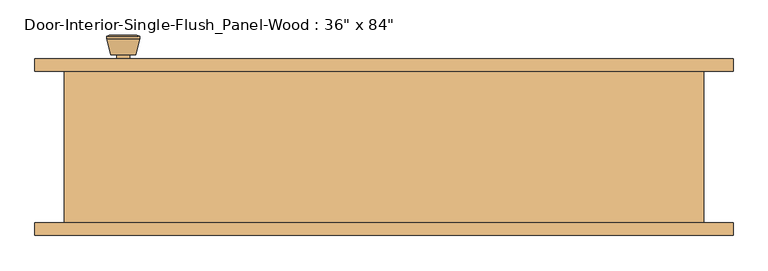
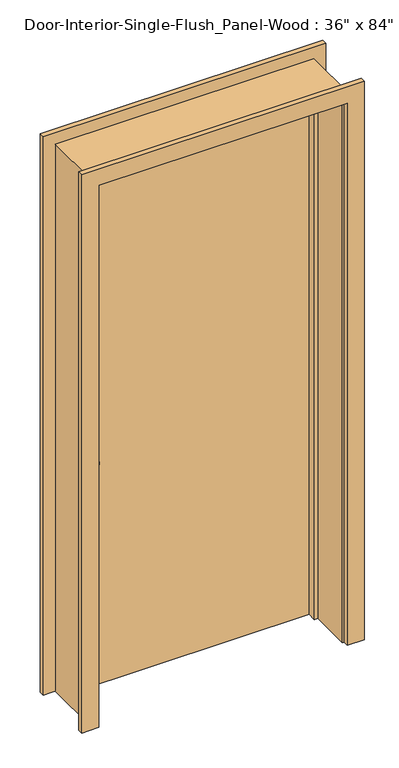
"""IFC4 building model written with IfcOpenShell, lengths in millimetres: door geometry."""

from ifc_helpers import new_model, si_unit, point, frame, frame_2d, origin, origin_with_axes, place, context, project, spatial, polyline, circle_curve, trimmed, segment, composite_curve, outline, extrude, faceted_brep, source, transform, mapped, element, save
from ifc_brep_helpers import plane_surface, cylinder_surface, revolved_surface, advanced_brep


def door_1d7b229f(model_context):
    return source(origin(), model_context, "Body", "SolidModel", [
        advanced_brep(
        [(-393.7, 70.2, 914.4), (-383.7, 70.2, 914.4), (-403.7, 70.2, 914.4), (-373.2241324, 21.2, 914.4), (-393.7, 21.2, 914.4), (-414.1758676, 21.2, 914.4), (-368.7, 23.0278681, 914.4), (-418.7, 23.0278681, 914.4), (-368.7, 26.4915463, 914.4), (-418.7, 26.4915463, 914.4), (-375.063764, 51.2, 914.4), (-412.336236, 51.2, 914.4), (-383.7, 51.2, 914.4), (-403.7, 51.2, 914.4)],
        [
            (0, 1),
            (1, 2, circle_curve(frame((-393.7, 70.2, 914.4), z_axis=(0.0, 1.0, 0.0), x_axis=(-1.0, 0.0, 0.0)), 10.0)),
            (2, 0),
            (2, 1, circle_curve(frame((-393.7, 70.2, 914.4), z_axis=(0.0, 1.0, 0.0), x_axis=(-1.0, 0.0, 0.0)), 10.0)),
            (3, 4),
            (4, 5),
            (5, 3, circle_curve(frame((-393.7, 21.2, 914.4), z_axis=(0.0, -1.0, 0.0), x_axis=(-1.0, 0.0, 0.0)), 20.4758676)),
            (3, 5, circle_curve(frame((-393.7, 21.2, 914.4), z_axis=(0.0, -1.0, 0.0), x_axis=(-1.0, 0.0, 0.0)), 20.4758676)),
            (6, 3),
            (5, 7),
            (7, 6, circle_curve(frame((-393.7, 23.0278681, 914.4), z_axis=(0.0, -1.0, 0.0), x_axis=(-1.0, 0.0, 0.0)), 25.0)),
            (6, 7, circle_curve(frame((-393.7, 23.0278681, 914.4), z_axis=(0.0, -1.0, 0.0), x_axis=(-1.0, 0.0, 0.0)), 25.0)),
            (8, 6),
            (7, 9),
            (9, 8, circle_curve(frame((-393.7, 26.4915463, 914.4), z_axis=(0.0, -1.0, 0.0), x_axis=(-1.0, 0.0, 0.0)), 25.0)),
            (8, 9, circle_curve(frame((-393.7, 26.4915463, 914.4), z_axis=(0.0, -1.0, 0.0), x_axis=(-1.0, 0.0, 0.0)), 25.0)),
            (10, 8),
            (9, 11),
            (11, 10, circle_curve(frame((-393.7, 51.2, 914.4), z_axis=(0.0, -1.0, 0.0), x_axis=(-1.0, 0.0, 0.0)), 18.636236)),
            (10, 11, circle_curve(frame((-393.7, 51.2, 914.4), z_axis=(0.0, -1.0, 0.0), x_axis=(-1.0, 0.0, 0.0)), 18.636236)),
            (12, 10),
            (11, 13),
            (13, 12, circle_curve(frame((-393.7, 51.2, 914.4), z_axis=(0.0, -1.0, 0.0), x_axis=(-1.0, 0.0, 0.0)), 10.0)),
            (12, 13, circle_curve(frame((-393.7, 51.2, 914.4), z_axis=(0.0, -1.0, 0.0), x_axis=(-1.0, 0.0, 0.0)), 10.0)),
            (1, 12),
            (13, 2),
        ],
        [
            plane_surface(frame((-393.7, 70.2, 914.4), z_axis=(0.0, 1.0, 0.0), x_axis=(-1.0, 0.0, 0.0))),
            plane_surface(frame((-393.7, 21.2, 914.4), z_axis=(0.0, -1.0, 0.0), x_axis=(-1.0, 0.0, 0.0))),
            revolved_surface(polyline([(-414.1758676, 21.2, 914.4), (-418.7, 23.0278681, 914.4)]), (-393.7, 70.2, 914.4), (0.0, 1.0, 0.0)),
            cylinder_surface(frame((-393.7, 70.2, 914.4), z_axis=(0.0, 1.0, 0.0), x_axis=(-1.0, 0.0, 0.0)), 25.0),
            revolved_surface(polyline([(-418.7, 26.4915463, 914.4), (-412.336236, 51.2, 914.4)]), (-393.7, 70.2, 914.4), (0.0, 1.0, 0.0)),
            plane_surface(frame((-393.7, 51.2, 914.4), z_axis=(0.0, 1.0, 0.0), x_axis=(-1.0, 0.0, 0.0))),
            cylinder_surface(frame((-393.7, 70.2, 914.4), z_axis=(0.0, 1.0, 0.0), x_axis=(-1.0, 0.0, 0.0)), 10.0),
        ],
        [
            (0, [[1, 2, 3]]),
            (0, [[-3, 4, -1]]),
            (1, [[5, 6, 7]]),
            (1, [[-6, -5, 8]]),
            (2, [[9, -7, 10, 11]]),
            (2, [[-10, -8, -9, 12]]),
            (3, [[13, -11, 14, 15]]),
            (3, [[-14, -12, -13, 16]]),
            (4, [[17, -15, 18, 19]]),
            (4, [[-18, -16, -17, 20]]),
            (5, [[21, -19, 22, 23]]),
            (5, [[-22, -20, -21, 24]]),
            (6, [[25, -23, 26, -2]]),
            (6, [[-26, -24, -25, -4]]),
        ],
    ),
        extrude(outline(composite_curve([segment(trimmed(circle_curve(frame_2d((914.4, -393.7)), 30.0), [point((914.4, -423.7))], [point((914.4, -363.7))], False, "CARTESIAN"), True, "CONTINUOUS"), segment(trimmed(circle_curve(frame_2d((914.4, -393.7)), 30.0), [point((914.4, -363.7))], [point((914.4, -423.7))], False, "CARTESIAN"), True, "CONTINUOUS")], self_intersect=False)), frame((0.0, 70.2, 0.0), z_axis=(0.0, 1.0, 0.0), x_axis=(0.0, 0.0, 1.0)), (0.0, 0.0, 1.0), 6.0),
        advanced_brep(
        [(-393.7, 117.125, 914.4), (-403.7, 117.125, 914.4), (-383.7, 117.125, 914.4), (-373.2241324, 166.125, 914.4), (-414.1758676, 166.125, 914.4), (-393.7, 166.125, 914.4), (-368.7, 164.2971319, 914.4), (-418.7, 164.2971319, 914.4), (-368.7, 160.8334537, 914.4), (-418.7, 160.8334537, 914.4), (-375.063764, 136.125, 914.4), (-412.336236, 136.125, 914.4), (-383.7, 136.125, 914.4), (-403.7, 136.125, 914.4)],
        [
            (0, 1),
            (1, 2, circle_curve(frame((-393.7, 117.125, 914.4), z_axis=(0.0, -1.0, 0.0), x_axis=(-1.0, 0.0, 0.0)), 10.0)),
            (2, 0),
            (2, 1, circle_curve(frame((-393.7, 117.125, 914.4), z_axis=(0.0, -1.0, 0.0), x_axis=(-1.0, 0.0, 0.0)), 10.0)),
            (3, 4, circle_curve(frame((-393.7, 166.125, 914.4), z_axis=(0.0, 1.0, 0.0), x_axis=(-1.0, 0.0, 0.0)), 20.4758676)),
            (4, 5),
            (5, 3),
            (4, 3, circle_curve(frame((-393.7, 166.125, 914.4), z_axis=(0.0, 1.0, 0.0), x_axis=(-1.0, 0.0, 0.0)), 20.4758676)),
            (6, 7, circle_curve(frame((-393.7, 164.2971319, 914.4), z_axis=(0.0, 1.0, 0.0), x_axis=(-1.0, 0.0, 0.0)), 25.0)),
            (7, 4),
            (3, 6),
            (7, 6, circle_curve(frame((-393.7, 164.2971319, 914.4), z_axis=(0.0, 1.0, 0.0), x_axis=(-1.0, 0.0, 0.0)), 25.0)),
            (8, 9, circle_curve(frame((-393.7, 160.8334537, 914.4), z_axis=(0.0, 1.0, 0.0), x_axis=(-1.0, 0.0, 0.0)), 25.0)),
            (9, 7),
            (6, 8),
            (9, 8, circle_curve(frame((-393.7, 160.8334537, 914.4), z_axis=(0.0, 1.0, 0.0), x_axis=(-1.0, 0.0, 0.0)), 25.0)),
            (10, 11, circle_curve(frame((-393.7, 136.125, 914.4), z_axis=(0.0, 1.0, 0.0), x_axis=(-1.0, 0.0, 0.0)), 18.636236)),
            (11, 9),
            (8, 10),
            (11, 10, circle_curve(frame((-393.7, 136.125, 914.4), z_axis=(0.0, 1.0, 0.0), x_axis=(-1.0, 0.0, 0.0)), 18.636236)),
            (12, 13, circle_curve(frame((-393.7, 136.125, 914.4), z_axis=(0.0, 1.0, 0.0), x_axis=(-1.0, 0.0, 0.0)), 10.0)),
            (13, 11),
            (10, 12),
            (13, 12, circle_curve(frame((-393.7, 136.125, 914.4), z_axis=(0.0, 1.0, 0.0), x_axis=(-1.0, 0.0, 0.0)), 10.0)),
            (1, 13),
            (12, 2),
        ],
        [
            plane_surface(frame((-393.7, 117.125, 914.4), z_axis=(0.0, -1.0, 0.0), x_axis=(-1.0, 0.0, 0.0))),
            plane_surface(frame((-393.7, 166.125, 914.4), z_axis=(0.0, 1.0, 0.0), x_axis=(-1.0, 0.0, 0.0))),
            revolved_surface(polyline([(-414.1758676, 166.125, 914.4), (-418.7, 164.2971319, 914.4)]), (-393.7, 117.125, 914.4), (0.0, -1.0, 0.0)),
            cylinder_surface(frame((-393.7, 117.125, 914.4), z_axis=(0.0, -1.0, 0.0), x_axis=(-1.0, 0.0, 0.0)), 25.0),
            revolved_surface(polyline([(-418.7, 160.8334537, 914.4), (-412.336236, 136.125, 914.4)]), (-393.7, 117.125, 914.4), (0.0, -1.0, 0.0)),
            plane_surface(frame((-393.7, 136.125, 914.4), z_axis=(0.0, -1.0, 0.0), x_axis=(-1.0, 0.0, 0.0))),
            cylinder_surface(frame((-393.7, 117.125, 914.4), z_axis=(0.0, -1.0, 0.0), x_axis=(-1.0, 0.0, 0.0)), 10.0),
        ],
        [
            (0, [[1, 2, 3]]),
            (0, [[-3, 4, -1]]),
            (1, [[5, 6, 7]]),
            (1, [[8, -7, -6]]),
            (2, [[9, 10, -5, 11]]),
            (2, [[12, -11, -8, -10]]),
            (3, [[13, 14, -9, 15]]),
            (3, [[16, -15, -12, -14]]),
            (4, [[17, 18, -13, 19]]),
            (4, [[20, -19, -16, -18]]),
            (5, [[21, 22, -17, 23]]),
            (5, [[24, -23, -20, -22]]),
            (6, [[-2, 25, -21, 26]]),
            (6, [[-4, -26, -24, -25]]),
        ],
    ),
        extrude(outline(composite_curve([segment(trimmed(circle_curve(frame_2d((914.4, -393.7)), 30.0), [point((914.4, -423.7))], [point((914.4, -363.7))], False, "CARTESIAN"), True, "CONTINUOUS"), segment(trimmed(circle_curve(frame_2d((914.4, -393.7)), 30.0), [point((914.4, -363.7))], [point((914.4, -423.7))], False, "CARTESIAN"), True, "CONTINUOUS")], self_intersect=False)), frame((0.0, 111.125, 0.0), z_axis=(0.0, 1.0, 0.0), x_axis=(0.0, 0.0, 1.0)), (0.0, 0.0, 1.0), 6.0),
        faceted_brep([(482.6, 111.125, 0.0), (482.6, -117.475, 0.0), (457.2, -117.475, 0.0), (457.2, 41.275, 0.0), (444.5, 41.275, 0.0), (444.5, 76.2, 0.0), (457.2, 76.2, 0.0), (457.2, 111.125, 0.0), (482.6, 111.125, 2159.0), (482.6, -117.475, 2159.0), (-482.6, -117.475, 2159.0), (-482.6, -117.475, 0.0), (-457.2, -117.475, 0.0), (-457.2, -117.475, 2133.6), (457.2, -117.475, 2133.6), (457.2, 41.275, 2133.6), (-457.2, 41.275, 2133.6), (-457.2, 41.275, 0.0), (-444.5, 41.275, 0.0), (-444.5, 41.275, 2120.9), (444.5, 41.275, 2120.9), (444.5, 76.2, 2120.9), (-444.5, 76.2, 2120.9), (-444.5, 76.2, 0.0), (-457.2, 76.2, 0.0), (-457.2, 76.2, 2133.6), (457.2, 76.2, 2133.6), (457.2, 111.125, 2133.6), (-457.2, 111.125, 2133.6), (-457.2, 111.125, 0.0), (-482.6, 111.125, 0.0), (-482.6, 111.125, 2159.0)], [[[0, 1, 2, 3, 4, 5, 6, 7]], [[1, 0, 8, 9]], [[2, 1, 9, 10, 11, 12, 13, 14]], [[3, 2, 14, 15]], [[4, 3, 15, 16, 17, 18, 19, 20]], [[5, 4, 20, 21]], [[6, 5, 21, 22, 23, 24, 25, 26]], [[7, 6, 26, 27]], [[0, 7, 27, 28, 29, 30, 31, 8]], [[9, 8, 31, 10]], [[15, 14, 13, 16]], [[21, 20, 19, 22]], [[27, 26, 25, 28]], [[30, 29, 24, 23, 18, 17, 12, 11]], [[10, 31, 30, 11]], [[16, 13, 12, 17]], [[22, 19, 18, 23]], [[28, 25, 24, 29]]]),
        extrude(outline(polyline([(457.2, 76.2), (-457.2, 76.2), (-457.2, 111.125), (457.2, 111.125), (457.2, 76.2)])), origin_with_axes(), (0.0, 0.0, 1.0), 2133.6),
        extrude(outline(polyline([(0.0, 463.55), (0.0, 527.05), (2203.45, 527.05), (2203.45, -527.05), (0.0, -527.05), (0.0, -463.55), (2139.95, -463.55), (2139.95, 463.55), (0.0, 463.55)])), frame((0.0, 111.125, 0.0), z_axis=(0.0, 1.0, 0.0), x_axis=(0.0, 0.0, 1.0)), (0.0, 0.0, 1.0), 19.05),
        extrude(outline(polyline([(0.0, 463.55), (0.0, 527.05), (2203.45, 527.05), (2203.45, -527.05), (0.0, -527.05), (0.0, -463.55), (2139.95, -463.55), (2139.95, 463.55), (0.0, 463.55)])), frame((0.0, -136.525, 0.0), z_axis=(0.0, 1.0, 0.0), x_axis=(0.0, 0.0, 1.0)), (0.0, 0.0, 1.0), 19.05),
    ])


if __name__ == "__main__":
    model = new_model("IFC4")
    model_context = context("Model", 3, world=origin())
    ifc_project = project(units=[si_unit("LENGTHUNIT", "METRE", prefix="MILLI")], contexts=[model_context])
    site = spatial("IfcSite", under=ifc_project)
    building = spatial("IfcBuilding", under=site)
    placement = place(None, origin())
    door_shape = door_1d7b229f(model_context)
    element("IfcDoor", 1, ObjectType="Door-Interior-Single-Flush_Panel-Wood : 36\" x 84\"", at=placement, inside=building, context=model_context, shape_type="MappedRepresentation", body=[
        mapped(door_shape, transform((0.0, 0.0, 0.0), x_axis=(1.0, 0.0, 0.0), y_axis=(0.0, 1.0, 0.0), z_axis=(0.0, 0.0, 1.0))),
    ])
    save(model, "model.ifc")

# Revit data of these elements
# Type "Door-Interior-Single-Flush_Panel-Wood : 36\" x 84\""
#   Type Mark = "12"
#   Analytic Construction = "Wooden"
#   Thickness = 0' - 1 3/8"
#   Thermal Resistance (R) = 2.5876 (h·ft²·°F)/BTU
#   Swing Angle [instance default] = 90.00°
#   Rough Width = 3' - 2"
#   Rough Height = 7' - 1"
#   Height = 7' - 0"
#   Width = 3' - 0"
#   Heat Transfer Coefficient (U) = 0.3865 BTU/(h·ft²·°F)
#   Trim Material = Cherry
#   Panel Material = Cherry
#   Frame Material = Cherry
#   Door Handle Material = Aluminum
#   Visual Light Transmittance = 0
#   Solar Heat Gain Coefficient = 0
#   Wall Closure = (empty or 0)
#   Function = (empty or 0)
# Element 1 (IfcDoor, "Door-Interior-Single-Flush_Panel-Wood : 36\" x 84\"")
#   Materials on its faces: "Cherry", "Aluminum"
# Materials
#   "Cherry": class "Wood", colour RGB 226 177 128, transparency 0, Description = "Prunus Serotina", Cost = 0
#   "Aluminum": class "Metal", colour RGB 247 247 247, transparency 0, Description = "Aluminum 6061", Cost = 0
